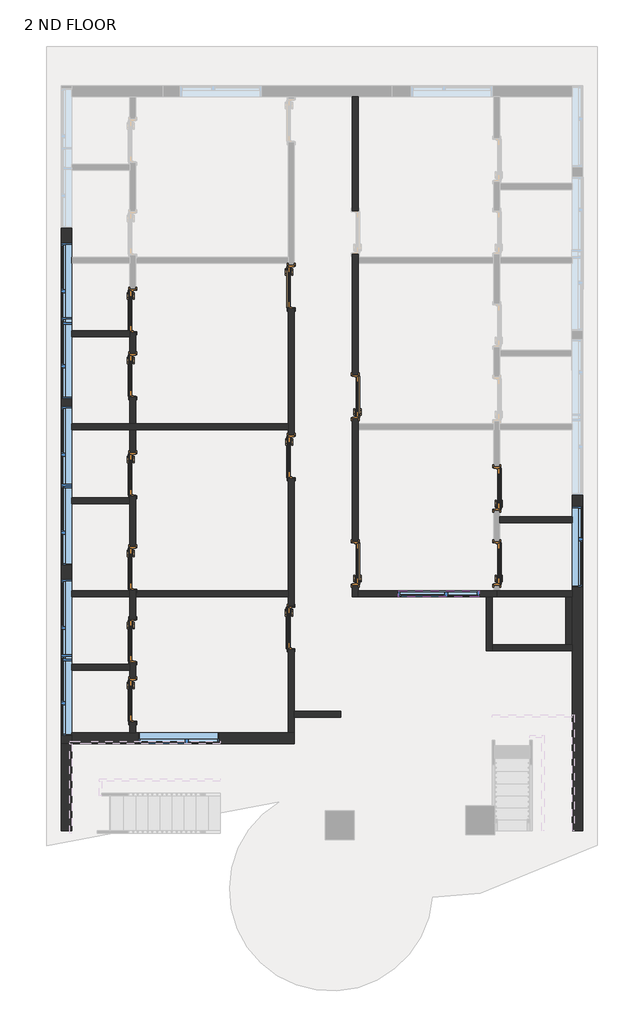
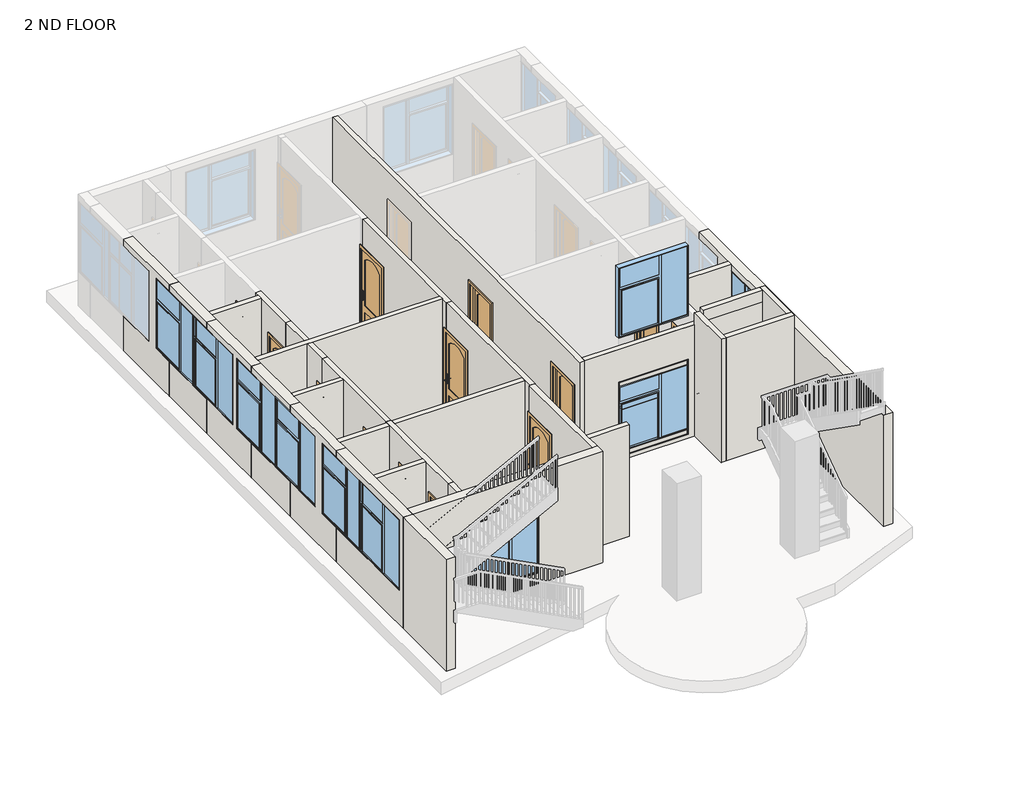
# One storey, part 1 of 4: 32 walls, 13 doors, 11 windows.
"""IFC4 building model written with IfcOpenShell, lengths in millimetres."""

from ifc_helpers import new_model, si_unit, frame, origin, place, context, project, spatial, polyline, outline, extrude, faceted_brep, transform, mapped, element, save
from components import door_346b4a94, m_window_casement_double_sidelight_1702_x_1829mm_c8b42c7f, m_window_casement_double_sidelight_1702_x_1829mm_92594323

model = new_model("IFC4")

# Units and contexts
model_context = context("Model", 3, world=origin())
ifc_project = project(units=[si_unit("LENGTHUNIT", "METRE", prefix="MILLI")], contexts=[model_context])

# Site, building, storey
site = spatial("IfcSite", under=ifc_project)
building = spatial("IfcBuilding", under=site)
storey = spatial("IfcBuildingStorey", under=building, Name="2 ND FLOOR", Elevation=6400.8)

# Doors
placement = place(None, origin())
door_shape = door_346b4a94(model_context)
element("IfcDoor", 1, ObjectType="2'10\"X7'", at=placement, inside=storey, context=model_context, shape_type="MappedRepresentation", body=[
    mapped(door_shape, transform((2698.7641134, -459.3600272, 6400.8), x_axis=(0.0, -1.0, 0.0), y_axis=(1.0, 0.0, 0.0), z_axis=(0.0, 0.0, 1.0))),
])
element("IfcDoor", 2, ObjectType="2'10\"X7'", at=placement, inside=storey, context=model_context, shape_type="MappedRepresentation", body=[
    mapped(door_shape, transform((2698.7641134, -2034.1600272, 6400.8), x_axis=(0.0, -1.0, 0.0), y_axis=(1.0, 0.0, 0.0), z_axis=(0.0, 0.0, 1.0))),
])
element("IfcDoor", 3, ObjectType="2'10\"X7'", at=placement, inside=storey, context=model_context, shape_type="MappedRepresentation", body=[
    mapped(door_shape, transform((-273.0358866, -2034.1600272, 6400.8), x_axis=(0.0, -1.0, 0.0), y_axis=(1.0, 0.0, 0.0), z_axis=(0.0, 0.0, 1.0))),
])
element("IfcDoor", 4, ObjectType="2'10\"X7'", at=placement, inside=storey, context=model_context, shape_type="MappedRepresentation", body=[
    mapped(door_shape, transform((-273.0358866, 1471.0399728, 6400.8), x_axis=(0.0, -1.0, 0.0), y_axis=(1.0, 0.0, 0.0), z_axis=(0.0, 0.0, 1.0))),
])
element("IfcDoor", 5, ObjectType="2'10\"X7'", at=placement, inside=storey, context=model_context, shape_type="MappedRepresentation", body=[
    mapped(door_shape, transform((-4952.9858866, -3659.7600272, 6400.8), x_axis=(0.0, 1.0, 0.0), y_axis=(-1.0, 0.0, 0.0), z_axis=(0.0, 0.0, 1.0))),
])
element("IfcDoor", 6, ObjectType="2'10\"X7'", at=placement, inside=storey, context=model_context, shape_type="MappedRepresentation", body=[
    mapped(door_shape, transform((-4952.9858866, -2142.5151651, 6400.8), x_axis=(0.0, 1.0, 0.0), y_axis=(-1.0, 0.0, 0.0), z_axis=(0.0, 0.0, 1.0))),
])
element("IfcDoor", 7, ObjectType="2'10\"X7'", at=placement, inside=storey, context=model_context, shape_type="MappedRepresentation", body=[
    mapped(door_shape, transform((-4952.9858866, -167.9704957, 6400.8), x_axis=(0.0, 1.0, 0.0), y_axis=(-1.0, 0.0, 0.0), z_axis=(0.0, 0.0, 1.0))),
])
element("IfcDoor", 8, ObjectType="2'10\"X7'", at=placement, inside=storey, context=model_context, shape_type="MappedRepresentation", body=[
    mapped(door_shape, transform((-4952.9858866, 3273.6174518, 6400.8), x_axis=(0.0, 1.0, 0.0), y_axis=(-1.0, 0.0, 0.0), z_axis=(0.0, 0.0, 1.0))),
])
element("IfcDoor", 9, ObjectType="2'10\"X7'", at=placement, inside=storey, context=model_context, shape_type="MappedRepresentation", body=[
    mapped(door_shape, transform((-1625.1621817, 3775.8008884, 6400.8), x_axis=(0.0, 1.0, 0.0), y_axis=(-1.0, 0.0, 0.0), z_axis=(0.0, 0.0, 1.0))),
])
element("IfcDoor", 10, ObjectType="2'10\"X7'", at=placement, inside=storey, context=model_context, shape_type="MappedRepresentation", body=[
    mapped(door_shape, transform((-1629.1419858, -3390.4626067, 6400.8), x_axis=(0.0, 1.0, 0.0), y_axis=(-1.0, 0.0, 0.0), z_axis=(0.0, 0.0, 1.0))),
])
element("IfcDoor", 11, ObjectType="2'10\"X7'", at=placement, inside=storey, context=model_context, shape_type="MappedRepresentation", body=[
    mapped(door_shape, transform((-1620.1577262, 202.9637706, 6400.8), x_axis=(0.0, 1.0, 0.0), y_axis=(-1.0, 0.0, 0.0), z_axis=(0.0, 0.0, 1.0))),
])
element("IfcDoor", 12, ObjectType="2'10\"X7'", at=placement, inside=storey, context=model_context, shape_type="MappedRepresentation", body=[
    mapped(door_shape, transform((-4952.9858866, -4917.0600272, 6400.8), x_axis=(0.0, 1.0, 0.0), y_axis=(-1.0, 0.0, 0.0), z_axis=(0.0, 0.0, 1.0))),
])
element("IfcDoor", 13, ObjectType="2'10\"X7'", at=placement, inside=storey, context=model_context, shape_type="MappedRepresentation", body=[
    mapped(door_shape, transform((-4952.9858866, 1913.3521609, 6400.8), x_axis=(0.0, 1.0, 0.0), y_axis=(-1.0, 0.0, 0.0), z_axis=(0.0, 0.0, 1.0))),
])

# Walls
element("IfcWall", 14, ObjectType="Generic - 4.5\"", at=placement, inside=storey, context=model_context, shape_type="Brep", body=[
    faceted_brep([(-6232.5508078, 2728.3399728, 6400.8), (-5013.3108866, 2728.3399728, 6400.8), (-5013.3108866, 2728.3399728, 9296.4), (-6232.5508078, 2728.3399728, 9296.4), (-6232.5508078, 2855.3399728, 6400.8), (-6232.5508078, 2855.3399728, 9296.4), (-5013.3108866, 2855.3399728, 9296.4), (-5013.3108866, 2855.3399728, 6400.8), (-5013.3108866, 2816.8174518, 6400.8)], [[[0, 1, 2, 3]], [[4, 5, 6, 7]], [[1, 0, 4, 7, 8]], [[0, 3, 5, 4]], [[2, 1, 8, 7, 6]], [[3, 2, 6, 5]]]),
])
element("IfcWall", 15, ObjectType="Generic - 4.5\"", at=placement, inside=storey, context=model_context, shape_type="Brep", body=[
    faceted_brep([(-5013.3108866, 2968.8174518, 9296.4), (-5013.3108866, 2968.8174518, 8559.4), (-5013.3108866, 2816.8174518, 8559.4), (-5013.3108866, 2816.8174518, 6400.8), (-5013.3108866, 2728.3399728, 6400.8), (-5013.3108866, 2370.1521609, 6400.8), (-5013.3108866, 2370.1521609, 8559.4), (-5013.3108866, 1684.7521609, 8559.4), (-5013.3108866, 1684.7521609, 9296.4), (-5013.3108866, 2728.3399728, 9296.4), (-5013.3108866, 2855.3399728, 9296.4), (-4886.3108866, 2968.8174518, 8559.4), (-4886.3108866, 2968.8174518, 9296.4), (-4886.3108866, 1684.7521609, 9296.4), (-4886.3108866, 1684.7521609, 8559.4), (-4886.3108866, 2370.1521609, 8559.4), (-4886.3108866, 2370.1521609, 6400.8), (-4886.3108866, 2816.8174518, 6400.8), (-4886.3108866, 2816.8174518, 8559.4)], [[[0, 1, 2, 3, 4, 5, 6, 7, 8, 9, 10]], [[11, 12, 13, 14, 15, 16, 17, 18]], [[3, 17, 16, 5, 4]], [[13, 8, 7, 14]], [[1, 0, 12, 11]], [[18, 2, 1, 11]], [[2, 18, 17, 3]], [[15, 6, 5, 16]], [[6, 15, 14, 7]], [[0, 10, 9, 8, 13, 12]]]),
])
element("IfcWall", 16, ObjectType="Generic - 4.5\"", at=placement, inside=storey, context=model_context, shape_type="Brep", body=[
    faceted_brep([(-6232.5508078, 772.5399728, 6400.8), (-5013.3108866, 772.5399728, 6400.8), (-4886.3108866, 772.5399728, 6400.8), (-1685.9108866, 772.5399728, 6400.8), (-1685.9108866, 772.5399728, 9296.4), (-4886.3108866, 772.5399728, 9296.4), (-5013.3108866, 772.5399728, 9296.4), (-6232.5508078, 772.5399728, 9296.4), (-6232.5508078, 899.5399728, 6400.8), (-6232.5508078, 899.5399728, 9296.4), (-5013.3108866, 899.5399728, 9296.4), (-4886.3108866, 899.5399728, 9296.4), (-1685.9108866, 899.5399728, 9296.4), (-1685.9108866, 899.5399728, 6400.8), (-4886.3108866, 899.5399728, 6400.8), (-5013.3108866, 899.5399728, 6400.8)], [[[0, 1, 2, 3, 4, 5, 6, 7]], [[8, 9, 10, 11, 12, 13, 14, 15]], [[3, 2, 1, 0, 8, 15, 14, 13]], [[4, 3, 13, 12]], [[0, 7, 9, 8]], [[7, 6, 5, 4, 12, 11, 10, 9]]]),
])
element("IfcWall", 17, ObjectType="Generic - 4.5\"", at=placement, inside=storey, context=model_context, shape_type="SweptSolid", body=[
    extrude(outline(polyline([(136.8295043, 8559.4), (136.8295043, 9296.4), (772.5399728, 9296.4), (772.5399728, 6400.8), (288.8295043, 6400.8), (288.8295043, 8559.4), (136.8295043, 8559.4)])), frame((-5013.3108866, 0.0, 0.0), z_axis=(1.0, 0.0, 0.0), x_axis=(0.0, 1.0, 0.0)), (0.0, 0.0, 1.0), 127.0),
    extrude(outline(polyline([(1684.7521609, 9296.4), (1684.7521609, 8559.4), (1456.5521609, 8559.4), (1456.5521609, 6400.8), (899.5399728, 6400.8), (899.5399728, 9296.4), (1684.7521609, 9296.4)])), frame((-5013.3108866, 0.0, 0.0), z_axis=(1.0, 0.0, 0.0), x_axis=(0.0, 1.0, 0.0)), (0.0, 0.0, 1.0), 127.0),
])
element("IfcWall", 18, ObjectType="Generic - 4.5\"", at=placement, inside=storey, context=model_context, shape_type="SweptSolid", body=[
    extrude(outline(polyline([(-5013.3108866, -776.8600272), (-6232.5508078, -776.8600272), (-6232.5508078, -649.8600272), (-5013.3108866, -649.8600272), (-5013.3108866, -776.8600272)])), frame((0.0, 0.0, 6400.8), z_axis=(0.0, 0.0, 1.0), x_axis=(1.0, 0.0, 0.0)), (0.0, 0.0, 1.0), 2895.6),
])
element("IfcWall", 19, ObjectType="Generic - 4.5\"", at=placement, inside=storey, context=model_context, shape_type="Brep", body=[
    faceted_brep([(-5013.3108866, -2574.3151651, 8559.4), (-5013.3108866, -2574.3151651, 9296.4), (-5013.3108866, -776.8600272, 9296.4), (-5013.3108866, -649.8600272, 9296.4), (-5013.3108866, 136.8295043, 9296.4), (-5013.3108866, 136.8295043, 8559.4), (-5013.3108866, -624.7704957, 8559.4), (-5013.3108866, -624.7704957, 6400.8), (-5013.3108866, -649.8600272, 6400.8), (-5013.3108866, -776.8600272, 6400.8), (-5013.3108866, -1685.7151651, 6400.8), (-5013.3108866, -1685.7151651, 8559.4), (-4886.3108866, -2574.3151651, 9296.4), (-4886.3108866, -2574.3151651, 8559.4), (-4886.3108866, -1685.7151651, 8559.4), (-4886.3108866, -1685.7151651, 6400.8), (-4886.3108866, -624.7704957, 6400.8), (-4886.3108866, -624.7704957, 8559.4), (-4886.3108866, 136.8295043, 8559.4), (-4886.3108866, 136.8295043, 9296.4)], [[[0, 1, 2, 3, 4, 5, 6, 7, 8, 9, 10, 11]], [[12, 13, 14, 15, 16, 17, 18, 19]], [[15, 10, 9, 8, 7, 16]], [[1, 0, 13, 12]], [[4, 19, 18, 5]], [[14, 11, 10, 15]], [[11, 14, 13, 0]], [[17, 6, 5, 18]], [[6, 17, 16, 7]], [[4, 3, 2, 1, 12, 19]]]),
])
element("IfcWall", 20, ObjectType="Generic - 4.5\"", at=placement, inside=storey, context=model_context, shape_type="SweptSolid", body=[
    extrude(outline(polyline([(-5013.3108866, -2732.6600272), (-6232.5508078, -2732.6600272), (-6232.5508078, -2605.6600272), (-5013.3108866, -2605.6600272), (-5013.3108866, -2732.6600272)])), frame((0.0, 0.0, 6400.8), z_axis=(0.0, 0.0, 1.0), x_axis=(1.0, 0.0, 0.0)), (0.0, 0.0, 1.0), 2895.6),
])
element("IfcWall", 21, ObjectType="Generic - 4.5\"", at=placement, inside=storey, context=model_context, shape_type="Brep", body=[
    faceted_brep([(-5013.3108866, -3202.9600272, 6400.8), (-5013.3108866, -3202.9600272, 8559.4), (-5013.3108866, -4116.5600272, 8559.4), (-5013.3108866, -4116.5600272, 6400.8), (-5013.3108866, -4155.0600272, 6400.8), (-5013.3108866, -4282.0600272, 6400.8), (-5013.3108866, -4460.2600272, 6400.8), (-5013.3108866, -4460.2600272, 8559.4), (-5013.3108866, -5221.8600272, 8559.4), (-5013.3108866, -5221.8600272, 9296.4), (-5013.3108866, -4282.0600272, 9296.4), (-5013.3108866, -4155.0600272, 9296.4), (-5013.3108866, -2732.6600272, 9296.4), (-5013.3108866, -2605.6600272, 9296.4), (-5013.3108866, -2574.3151651, 9296.4), (-5013.3108866, -2574.3151651, 8559.4), (-5013.3108866, -2599.3151651, 8559.4), (-5013.3108866, -2599.3151651, 6400.8), (-5013.3108866, -2605.6600272, 6400.8), (-5013.3108866, -2732.6600272, 6400.8), (-4886.3108866, -3202.9600272, 8559.4), (-4886.3108866, -3202.9600272, 6400.8), (-4886.3108866, -2732.6600272, 6400.8), (-4886.3108866, -2605.6600272, 6400.8), (-4886.3108866, -2599.3151651, 6400.8), (-4886.3108866, -2599.3151651, 8559.4), (-4886.3108866, -2574.3151651, 8559.4), (-4886.3108866, -2574.3151651, 9296.4), (-4886.3108866, -2605.6600272, 9296.4), (-4886.3108866, -2732.6600272, 9296.4), (-4886.3108866, -5221.8600272, 9296.4), (-4886.3108866, -5221.8600272, 8559.4), (-4886.3108866, -4460.2600272, 8559.4), (-4886.3108866, -4460.2600272, 6400.8), (-4886.3108866, -4116.5600272, 6400.8), (-4886.3108866, -4116.5600272, 8559.4)], [[[0, 1, 2, 3, 4, 5, 6, 7, 8, 9, 10, 11, 12, 13, 14, 15, 16, 17, 18, 19]], [[20, 21, 22, 23, 24, 25, 26, 27, 28, 29, 30, 31, 32, 33, 34, 35]], [[21, 0, 19, 18, 17, 24, 23, 22]], [[3, 34, 33, 6, 5, 4]], [[30, 9, 8, 31]], [[15, 14, 27, 26]], [[20, 1, 0, 21]], [[1, 20, 35, 2]], [[2, 35, 34, 3]], [[25, 16, 15, 26]], [[16, 25, 24, 17]], [[32, 7, 6, 33]], [[7, 32, 31, 8]], [[14, 13, 12, 11, 10, 9, 30, 29, 28, 27]]]),
])
element("IfcWall", 22, ObjectType="Generic - 4.5\"", at=placement, inside=storey, context=model_context, shape_type="SweptSolid", body=[
    extrude(outline(polyline([(-5013.3108866, -4282.0600272), (-6232.5324766, -4282.0600272), (-6232.5342541, -4155.0600272), (-5013.3108866, -4155.0600272), (-5013.3108866, -4282.0600272)])), frame((0.0, 0.0, 6400.8), z_axis=(0.0, 0.0, 1.0), x_axis=(1.0, 0.0, 0.0)), (0.0, 0.0, 1.0), 2895.6),
])
element("IfcWall", 23, ObjectType="Generic - 4.5\"", at=placement, inside=storey, context=model_context, shape_type="SweptSolid", body=[
    extrude(outline(polyline([(-1685.9108866, -2732.6600272), (-4886.3108866, -2732.6600272), (-4886.3108866, -2605.6600272), (-1685.9108866, -2605.6600272), (-1685.9108866, -2732.6600272)])), frame((0.0, 0.0, 6400.8), z_axis=(0.0, 0.0, 1.0), x_axis=(1.0, 0.0, 0.0)), (0.0, 0.0, 1.0), 2895.6),
])
element("IfcWall", 24, ObjectType="Generic - 4.5\"", at=placement, inside=storey, context=model_context, shape_type="Brep", body=[
    faceted_brep([(-1685.4871817, 4182.2008884, 9296.4), (-1685.4871817, 4182.2008884, 8559.4), (-1685.4871817, 3319.0008884, 8559.4), (-1685.4871817, 3319.0008884, 6400.8), (-1685.4871817, 659.7637706, 6400.8), (-1685.4871817, 659.7637706, 8559.4), (-1685.4871817, 609.3637706, 8559.4), (-1685.4871817, 609.3637706, 9296.4), (-1558.4871817, 4182.2008884, 8559.4), (-1558.4871817, 4182.2008884, 9296.4), (-1558.4871817, 609.3637706, 9296.4), (-1558.4871817, 609.3637706, 8559.4), (-1558.4871817, 659.7637706, 8559.4), (-1558.4871817, 659.7637706, 6400.8), (-1558.4871817, 3319.0008884, 6400.8), (-1558.4871817, 3319.0008884, 8559.4), (-1680.4827262, 609.3637706, 9296.4), (-1680.4827262, 609.3637706, 8559.4), (-1558.9108866, 4182.2008884, 9296.4), (-1558.9108866, 4182.2008884, 8559.4)], [[[0, 1, 2, 3, 4, 5, 6, 7]], [[8, 9, 10, 11, 12, 13, 14, 15]], [[3, 14, 13, 4]], [[10, 16, 7, 6, 17, 11]], [[1, 0, 18, 9, 8, 19]], [[15, 2, 1, 19, 8]], [[2, 15, 14, 3]], [[12, 5, 4, 13]], [[5, 12, 11, 17, 6]], [[0, 7, 16, 10, 9, 18]]]),
])
element("IfcWall", 25, ObjectType="Generic - 4.5\"", at=placement, inside=storey, context=model_context, shape_type="Brep", body=[
    faceted_brep([(-1680.4827262, -2933.2626067, 6400.8), (-1680.4827262, -2933.2626067, 9296.4), (-1680.4827262, 609.3637706, 9296.4), (-1680.4827262, 609.3637706, 8559.4), (-1680.4827262, -253.8362294, 8559.4), (-1680.4827262, -253.8362294, 6400.8), (-1553.4827262, -2933.2626067, 9296.4), (-1553.4827262, -2933.2626067, 6400.8), (-1553.4827262, -253.8362294, 6400.8), (-1553.4827262, -253.8362294, 8559.4), (-1553.4827262, 609.3637706, 8559.4), (-1553.4827262, 609.3637706, 9296.4), (-1562.4669858, -2933.2626067, 6400.8), (-1562.4669858, -2933.2626067, 9296.4), (-1558.4871817, 609.3637706, 9296.4), (-1558.4871817, 609.3637706, 8559.4)], [[[0, 1, 2, 3, 4, 5]], [[6, 7, 8, 9, 10, 11]], [[7, 12, 0, 5, 8]], [[1, 0, 12, 7, 6, 13]], [[2, 14, 11, 10, 15, 3]], [[9, 4, 3, 15, 10]], [[4, 9, 8, 5]], [[2, 1, 13, 6, 11, 14]]]),
])
element("IfcWall", 26, ObjectType="Generic - 4.5\"", at=placement, inside=storey, context=model_context, shape_type="Brep", body=[
    faceted_brep([(-1689.4669858, -2933.2626067, 9296.4), (-1689.4669858, -2933.2626067, 6400.8), (-1689.4669858, -2933.6626067, 6400.8), (-1689.4669858, -2933.6626067, 8559.4), (-1689.4669858, -3847.2626067, 8559.4), (-1689.4669858, -3847.2626067, 6400.8), (-1689.4669858, -5596.1082131, 6400.8), (-1689.4669858, -5596.1082131, 9296.4), (-1562.4669858, -2933.2626067, 6400.8), (-1562.4669858, -2933.2626067, 9296.4), (-1562.4669858, -5136.3822004, 9296.4), (-1562.4669858, -5263.3822004, 9296.4), (-1562.4669858, -5596.1082131, 9296.4), (-1562.4669858, -5596.1082131, 6400.8), (-1562.4669858, -5263.3822004, 6400.8), (-1562.4669858, -5136.3822004, 6400.8), (-1562.4669858, -3847.2626067, 6400.8), (-1562.4669858, -3847.2626067, 8559.4), (-1562.4669858, -2933.6626067, 8559.4), (-1562.4669858, -2933.6626067, 6400.8), (-1680.4827262, -2933.2626067, 6400.8), (-1680.4827262, -2933.2626067, 9296.4)], [[[0, 1, 2, 3, 4, 5, 6, 7]], [[8, 9, 10, 11, 12, 13, 14, 15, 16, 17, 18, 19]], [[1, 20, 8, 19, 2]], [[13, 6, 5, 16, 15, 14]], [[1, 0, 21, 9, 8, 20]], [[18, 3, 2, 19]], [[3, 18, 17, 4]], [[4, 17, 16, 5]], [[7, 6, 13, 12]], [[0, 7, 12, 11, 10, 9, 21]]]),
])
element("IfcWall", 27, ObjectType="Generic - 4.5\"", at=placement, inside=storey, context=model_context, shape_type="Brep", body=[
    faceted_brep([(-339.7108866, 7782.9399728, 9296.4), (-339.7108866, 7782.9399728, 6400.8), (-339.7108866, 5382.2399728, 6400.8), (-339.7108866, 5382.2399728, 8559.4), (-339.7108866, 4468.6399728, 8559.4), (-339.7108866, 4468.6399728, 6400.8), (-339.7108866, 1927.8399728, 6400.8), (-339.7108866, 1927.8399728, 8559.4), (-339.7108866, 1014.2399728, 8559.4), (-339.7108866, 1014.2399728, 6400.8), (-339.7108866, -1577.3600272, 6400.8), (-339.7108866, -1577.3600272, 8559.4), (-339.7108866, -2490.9600272, 8559.4), (-339.7108866, -2490.9600272, 6400.8), (-339.7108866, -2732.6600272, 6400.8), (-339.7108866, -2732.6600272, 9296.4), (-212.7108866, 7782.9399728, 6400.8), (-212.7108866, 7782.9399728, 9296.4), (-212.7108866, 4404.7399728, 9296.4), (-212.7108866, 4277.7399728, 9296.4), (-212.7108866, 899.5399728, 9296.4), (-212.7108866, 772.5399728, 9296.4), (-212.7108866, -2605.6600272, 9296.4), (-212.7108866, -2732.6600272, 9296.4), (-212.7108866, -2732.6600272, 6400.8), (-212.7108866, -2605.6600272, 6400.8), (-212.7108866, -2490.9600272, 6400.8), (-212.7108866, -2490.9600272, 8559.4), (-212.7108866, -1577.3600272, 8559.4), (-212.7108866, -1577.3600272, 6400.8), (-212.7108866, 772.5399728, 6400.8), (-212.7108866, 899.5399728, 6400.8), (-212.7108866, 1014.2399728, 6400.8), (-212.7108866, 1014.2399728, 8559.4), (-212.7108866, 1927.8399728, 8559.4), (-212.7108866, 1927.8399728, 6400.8), (-212.7108866, 4277.7399728, 6400.8), (-212.7108866, 4404.7399728, 6400.8), (-212.7108866, 4468.6399728, 6400.8), (-212.7108866, 4468.6399728, 8559.4), (-212.7108866, 5382.2399728, 8559.4), (-212.7108866, 5382.2399728, 6400.8)], [[[0, 1, 2, 3, 4, 5, 6, 7, 8, 9, 10, 11, 12, 13, 14, 15]], [[16, 17, 18, 19, 20, 21, 22, 23, 24, 25, 26, 27, 28, 29, 30, 31, 32, 33, 34, 35, 36, 37, 38, 39, 40, 41]], [[1, 16, 41, 2]], [[24, 14, 13, 26, 25]], [[29, 10, 9, 32, 31, 30]], [[35, 6, 5, 38, 37, 36]], [[1, 0, 17, 16]], [[15, 14, 24, 23]], [[12, 27, 26, 13]], [[27, 12, 11, 28]], [[28, 11, 10, 29]], [[8, 33, 32, 9]], [[33, 8, 7, 34]], [[34, 7, 6, 35]], [[4, 39, 38, 5]], [[39, 4, 3, 40]], [[40, 3, 2, 41]], [[0, 15, 23, 22, 21, 20, 19, 18, 17]]]),
])
element("IfcWall", 28, ObjectType="Generic - 4.5\"", at=placement, inside=storey, context=model_context, shape_type="Brep", body=[
    faceted_brep([(-212.7108866, -2732.6600272, 6400.8), (2479.6891134, -2732.6600272, 6400.8), (2606.6891134, -2732.6600272, 6400.8), (4281.7311655, -2732.6600272, 6400.8), (4281.7311655, -2732.6600272, 9296.4), (-212.7108866, -2732.6600272, 9296.4), (625.4891134, -2732.6600272, 8454.7930467), (2327.2891134, -2732.6600272, 8454.7930467), (2327.2891134, -2732.6600272, 6625.9930467), (625.4891134, -2732.6600272, 6625.9930467), (-212.7108866, -2605.6600272, 6400.8), (-212.7108866, -2605.6600272, 9296.4), (2632.0891134, -2605.6600272, 9296.4), (2759.0891134, -2605.6600272, 9296.4), (4281.7311655, -2605.6600272, 9296.4), (4281.7311655, -2605.6600272, 6400.8), (2759.0891134, -2605.6600272, 6400.8), (2632.0891134, -2605.6600272, 6400.8), (625.4891134, -2605.6600272, 8454.7930467), (625.4891134, -2605.6600272, 6625.9930467), (2327.2891134, -2605.6600272, 6625.9930467), (2327.2891134, -2605.6600272, 8454.7930467)], [[[0, 1, 2, 3, 4, 5], [6, 7, 8, 9]], [[10, 11, 12, 13, 14, 15, 16, 17], [18, 19, 20, 21]], [[3, 2, 1, 0, 10, 17, 16, 15]], [[0, 5, 11, 10]], [[4, 3, 15, 14]], [[5, 4, 14, 13, 12, 11]], [[19, 18, 6, 9]], [[20, 19, 9, 8]], [[21, 20, 8, 7]], [[18, 21, 7, 6]]]),
])
element("IfcWall", 29, ObjectType="Generic - 4.5\"", at=placement, inside=storey, context=model_context, shape_type="SweptSolid", body=[
    extrude(outline(polyline([(4281.7311655, -1183.2600272), (2759.0891134, -1183.2600272), (2759.0891134, -1056.2600272), (4281.7311655, -1056.2600272), (4281.7311655, -1183.2600272)])), frame((0.0, 0.0, 6400.8), z_axis=(0.0, 0.0, 1.0), x_axis=(1.0, 0.0, 0.0)), (0.0, 0.0, 1.0), 2895.6),
])
element("IfcWall", 30, ObjectType="Generic - 4.5\"", at=placement, inside=storey, context=model_context, shape_type="Brep", body=[
    faceted_brep([(-212.7108866, -2732.6600272, 6400.8), (2479.6891134, -2732.6600272, 6400.8), (2606.6891134, -2732.6600272, 6400.8), (2695.5891134, -2732.6600272, 6400.8), (2695.5891134, -2732.6600272, 9296.4), (-212.7108866, -2732.6600272, 9296.4), (625.4891134, -2732.6600272, 8326.7883506), (2327.2891134, -2732.6600272, 8326.7883506), (2327.2891134, -2732.6600272, 6497.9883506), (625.4891134, -2732.6600272, 6497.9883506), (-212.7108866, -2605.6600272, 6400.8), (-212.7108866, -2605.6600272, 9296.4), (2632.0891134, -2605.6600272, 9296.4), (2695.5891134, -2605.6600272, 9296.4), (2695.5891134, -2605.6600272, 6400.8), (2632.0891134, -2605.6600272, 6400.8), (625.4891134, -2605.6600272, 8326.7883506), (625.4891134, -2605.6600272, 6497.9883506), (2327.2891134, -2605.6600272, 6497.9883506), (2327.2891134, -2605.6600272, 8326.7883506)], [[[0, 1, 2, 3, 4, 5], [6, 7, 8, 9]], [[10, 11, 12, 13, 14, 15], [16, 17, 18, 19]], [[3, 2, 1, 0, 10, 15, 14]], [[4, 3, 14, 13]], [[5, 4, 13, 12, 11]], [[17, 16, 6, 9]], [[18, 17, 9, 8]], [[19, 18, 8, 7]], [[16, 19, 7, 6]], [[0, 5, 11, 10]]]),
])
element("IfcWall", 31, ObjectType="Generic - 5\"", at=placement, inside=storey, context=model_context, shape_type="SweptSolid", body=[
    extrude(outline(polyline([(-5593.5822004, 6400.8), (-5593.5822004, 9296.4), (-5221.8600272, 9296.4), (-5221.8600272, 8559.4), (-5373.8600272, 8559.4), (-5373.8600272, 6400.8), (-5593.5822004, 6400.8)])), frame((-5013.3108866, 0.0, 0.0), z_axis=(1.0, 0.0, 0.0), x_axis=(0.0, 1.0, 0.0)), (0.0, 0.0, 1.0), 127.0),
])
element("IfcWall", 32, ObjectType="Generic - 5\"", at=placement, inside=storey, context=model_context, shape_type="SweptSolid", body=[
    extrude(outline(polyline([(-1562.4669858, -5136.3822004), (-581.0108866, -5136.3822004), (-581.0108866, -5263.3822004), (-1562.4669858, -5263.3822004), (-1562.4669858, -5136.3822004)])), frame((0.0, 0.0, 6400.8), z_axis=(0.0, 0.0, 1.0), x_axis=(1.0, 0.0, 0.0)), (0.0, 0.0, 1.0), 2895.6),
])
element("IfcWall", 33, ObjectType="Generic - 5\"", at=placement, inside=storey, context=model_context, shape_type="Brep", body=[
    faceted_brep([(2479.6891134, -2732.6600272, 6400.8), (2479.6891134, -3866.3822004, 6400.8), (2479.6891134, -3866.3822004, 9601.2), (2479.6891134, -2732.6600272, 9601.2), (2606.6891134, -2732.6600272, 6400.8), (2606.6891134, -2732.6600272, 9601.2), (2606.6891134, -3739.3822004, 9601.2), (2606.6891134, -3866.3822004, 9601.2), (2606.6891134, -3866.3822004, 6400.8), (2606.6891134, -3739.3822004, 6400.8)], [[[0, 1, 2, 3]], [[4, 5, 6, 7, 8, 9]], [[1, 0, 4, 9, 8]], [[3, 2, 7, 6, 5]], [[0, 3, 5, 4]], [[2, 1, 8, 7]]]),
])
element("IfcWall", 34, ObjectType="Generic - 5\"", at=placement, inside=storey, context=model_context, shape_type="Brep", body=[
    faceted_brep([(2606.6891134, -3866.3822004, 6400.8), (4281.7311655, -3866.3822004, 6400.8), (4281.7311655, -3866.3822004, 9601.2), (2606.6891134, -3866.3822004, 9601.2), (2606.6891134, -3739.3822004, 6400.8), (2606.6891134, -3739.3822004, 9601.2), (4154.7311655, -3739.3822004, 9601.2), (4281.7311655, -3739.3822004, 9601.2), (4281.7311655, -3739.3822004, 6400.8), (4154.7311655, -3739.3822004, 6400.8)], [[[0, 1, 2, 3]], [[4, 5, 6, 7, 8, 9]], [[1, 0, 4, 9, 8]], [[3, 2, 7, 6, 5]], [[0, 3, 5, 4]], [[2, 1, 8, 7]]]),
])
element("IfcWall", 35, ObjectType="Generic - 5\"", at=placement, inside=storey, context=model_context, shape_type="Brep", body=[
    faceted_brep([(4281.7311655, -3739.3822004, 6400.8), (4281.7311655, -2605.6600272, 6400.8), (4281.7311655, -2605.6600272, 9601.2), (4281.7311655, -3739.3822004, 9601.2), (4154.7311655, -3739.3822004, 6400.8), (4154.7311655, -3739.3822004, 9601.2), (4154.7311655, -2732.6600272, 9601.2), (4154.7311655, -2605.6600272, 9601.2), (4154.7311655, -2605.6600272, 6400.8), (4154.7311655, -2732.6600272, 6400.8)], [[[0, 1, 2, 3]], [[4, 5, 6, 7, 8, 9]], [[1, 0, 4, 9, 8]], [[3, 2, 7, 6, 5]], [[0, 3, 5, 4]], [[1, 8, 7, 2]]]),
])
element("IfcWall", 36, ObjectType="Generic - 5\"", at=placement, inside=storey, context=model_context, shape_type="Brep", body=[
    faceted_brep([(2695.5891134, -2732.6600272, 6400.8), (4154.7311655, -2732.6600272, 6400.8), (4154.7311655, -2732.6600272, 9601.2), (2695.5891134, -2732.6600272, 9601.2), (2695.5891134, -2732.6600272, 9296.4), (2695.5891134, -2605.6600272, 6400.8), (2695.5891134, -2605.6600272, 9296.4), (2695.5891134, -2605.6600272, 9601.2), (4154.7311655, -2605.6600272, 9601.2), (4154.7311655, -2605.6600272, 6400.8), (2759.0891134, -2605.6600272, 6400.8)], [[[0, 1, 2, 3, 4]], [[5, 6, 7, 8, 9, 10]], [[1, 0, 5, 10, 9]], [[3, 2, 8, 7]], [[0, 4, 3, 7, 6, 5]], [[2, 1, 9, 8]]]),
])
element("IfcWall", 37, ObjectType="Generic - 9\"", at=placement, inside=storey, context=model_context, shape_type="Brep", body=[
    faceted_brep([(4281.7311655, 200.5184135, 6400.8), (4281.7311655, -1056.2600272, 6400.8), (4281.7311655, -1183.2600272, 6400.8), (4281.7311655, -2605.6600272, 6400.8), (4281.7311655, -2732.6600272, 6400.8), (4281.7311655, -7650.9822004, 6400.8), (4281.7311655, -7650.9822004, 9296.4), (4281.7311655, -2732.6600272, 9296.4), (4281.7311655, -2605.6600272, 9296.4), (4281.7311655, -1183.2600272, 9296.4), (4281.7311655, -1056.2600272, 9296.4), (4281.7311655, 200.5184135, 9296.4), (4281.7311655, 200.5184135, 9129.6), (4281.7311655, -599.0600272, 9129.6), (4281.7311655, -599.0600272, 7300.8), (4281.7311655, 200.5184135, 7300.8), (4281.7311655, -2537.537179, 7300.8), (4281.7311655, -835.737179, 7300.8), (4281.7311655, -835.737179, 9129.6), (4281.7311655, -2537.537179, 9129.6), (4510.3311655, -7650.9822004, 6400.8), (4510.3311655, 200.5184135, 6400.8), (4510.3311655, 200.5184135, 7300.8), (4510.3311655, -599.0600272, 7300.8), (4510.3311655, -599.0600272, 9129.6), (4510.3311655, 200.5184135, 9129.6), (4510.3311655, 200.5184135, 9296.4), (4510.3311655, -7650.9822004, 9296.4), (4510.3311655, -835.737179, 7300.8), (4510.3311655, -2537.537179, 7300.8), (4510.3311655, -2537.537179, 9129.6), (4510.3311655, -835.737179, 9129.6), (4283.0918814, 200.5184135, 6400.8), (4283.0918814, 200.5184135, 7300.8), (4283.0918814, 200.5184135, 9296.4), (4283.0918814, 200.5184135, 9129.6)], [[[0, 1, 2, 3, 4, 5, 6, 7, 8, 9, 10, 11, 12, 13, 14, 15], [16, 17, 18, 19]], [[20, 21, 22, 23, 24, 25, 26, 27], [28, 29, 30, 31]], [[5, 4, 3, 2, 1, 0, 32, 21, 20]], [[6, 5, 20, 27]], [[21, 32, 0, 15, 33, 22]], [[12, 11, 34, 26, 25, 35]], [[13, 24, 23, 14]], [[14, 23, 22, 33, 15]], [[24, 13, 12, 35, 25]], [[28, 17, 16, 29]], [[17, 28, 31, 18]], [[18, 31, 30, 19]], [[29, 16, 19, 30]], [[11, 10, 9, 8, 7, 6, 27, 26, 34]]]),
])
element("IfcWall", 38, ObjectType="Generic - 9\"", at=placement, inside=storey, context=model_context, shape_type="Brep", body=[
    faceted_brep([(-6232.5108866, -5824.7082131, 6400.8), (-6232.5140859, -5596.1082131, 6400.8), (-6232.5324766, -4282.0600272, 6400.8), (-6232.5342541, -4155.0600272, 6400.8), (-6232.5508078, -2972.263382, 6400.8), (-6232.5508078, -2972.263382, 7300.8), (-6232.5131972, -5659.6082132, 7300.8), (-6232.5131972, -5659.6082132, 9129.6), (-6232.5508078, -2972.263382, 9129.6), (-6232.5508078, -2972.263382, 9296.4), (-6232.5342541, -4155.0600272, 9296.4), (-6232.5324766, -4282.0600272, 9296.4), (-6232.5140859, -5596.1082131, 9296.4), (-6232.5108866, -5824.7082131, 9296.4), (-6461.1508078, -2972.2665814, 6400.8), (-6461.1108866, -5824.7082131, 6400.8), (-6461.1108866, -5824.7082131, 9296.4), (-6461.1508078, -2972.2665814, 9296.4), (-6461.1508078, -2972.2665814, 9129.6), (-6461.1131972, -5659.6114126, 9129.6), (-6461.1131972, -5659.6114126, 7300.8), (-6461.1508078, -2972.2665814, 7300.8)], [[[0, 1, 2, 3, 4, 5, 6, 7, 8, 9, 10, 11, 12, 13]], [[14, 15, 16, 17, 18, 19, 20, 21]], [[4, 3, 2, 1, 0, 15, 14]], [[4, 14, 21, 5]], [[9, 8, 18, 17]], [[5, 21, 20, 6]], [[18, 8, 7, 19]], [[19, 7, 6, 20]], [[0, 13, 16, 15]], [[13, 12, 11, 10, 9, 17, 16]]]),
])
element("IfcWall", 39, ObjectType="Generic - 9\"", at=placement, inside=storey, context=model_context, shape_type="Brep", body=[
    faceted_brep([(-6232.5508078, -2972.2649817, 6400.8), (-6232.5508078, -2732.6600272, 6400.8), (-6232.5508078, -2605.6600272, 6400.8), (-6232.5508078, -1019.7048138, 6400.8), (-6232.5508078, -1019.7048138, 7300.8), (-6232.5508078, -2073.8048138, 7300.8), (-6232.5508078, -2073.8048138, 9129.6), (-6232.5508078, -1019.7048138, 9129.6), (-6232.5508078, -1019.7048138, 9296.4), (-6232.5508078, -2605.6600272, 9296.4), (-6232.5508078, -2732.6600272, 9296.4), (-6232.5508078, -2972.2649817, 9296.4), (-6232.5508078, -2972.2649817, 9129.6), (-6232.5508078, -2375.3633819, 9129.6), (-6232.5508078, -2375.3633819, 7300.8), (-6232.5508078, -2972.2649817, 7300.8), (-6461.1508078, -1019.7048138, 6400.8), (-6461.1508078, -2972.2649817, 6400.8), (-6461.1508078, -2972.2649817, 7300.8), (-6461.1508078, -2375.3665813, 7300.8), (-6461.1508078, -2375.3665813, 9129.6), (-6461.1508078, -2972.2649817, 9129.6), (-6461.1508078, -2972.2649817, 9296.4), (-6461.1508078, -1019.7048138, 9296.4), (-6461.1508078, -1019.7048138, 9129.6), (-6461.1508078, -2073.8048138, 9129.6), (-6461.1508078, -2073.8048138, 7300.8), (-6461.1508078, -1019.7048138, 7300.8)], [[[0, 1, 2, 3, 4, 5, 6, 7, 8, 9, 10, 11, 12, 13, 14, 15]], [[16, 17, 18, 19, 20, 21, 22, 23, 24, 25, 26, 27]], [[3, 2, 1, 0, 17, 16]], [[3, 16, 27, 4]], [[8, 7, 24, 23]], [[17, 0, 15, 18]], [[11, 22, 21, 12]], [[26, 5, 4, 27]], [[5, 26, 25, 6]], [[6, 25, 24, 7]], [[13, 20, 19, 14]], [[14, 19, 18, 15]], [[20, 13, 12, 21]], [[11, 10, 9, 8, 23, 22]]]),
])
element("IfcWall", 40, ObjectType="Generic - 9\"", at=placement, inside=storey, context=model_context, shape_type="Brep", body=[
    faceted_brep([(-6232.5508078, -1019.7048138, 6400.8), (-6232.5508078, -776.8600272, 6400.8), (-6232.5508078, -649.8600272, 6400.8), (-6232.5508078, 642.0011338, 6400.8), (-6232.5508078, 642.0011338, 7300.8), (-6232.5508078, -1019.7048138, 7300.8), (-6461.1508078, 642.0011338, 6400.8), (-6461.1508078, -1019.7048138, 6400.8), (-6461.1508078, -1019.7048138, 7300.8), (-6461.1508078, 642.0011338, 7300.8)], [[[0, 1, 2, 3, 4, 5]], [[6, 7, 8, 9]], [[3, 2, 1, 0, 7, 6]], [[3, 6, 9, 4]], [[7, 0, 5, 8]], [[4, 9, 8, 5]]]),
    faceted_brep([(-6232.5508078, -1019.7048138, 9129.6), (-6232.5508078, 642.0011338, 9129.6), (-6232.5508078, 642.0011338, 9296.4), (-6232.5508078, -649.8600272, 9296.4), (-6232.5508078, -776.8600272, 9296.4), (-6232.5508078, -1019.7048138, 9296.4), (-6461.1508078, 642.0011338, 9296.4), (-6461.1508078, 642.0011338, 9129.6), (-6461.1508078, -1019.7048138, 9129.6), (-6461.1508078, -1019.7048138, 9296.4)], [[[0, 1, 2, 3, 4, 5]], [[6, 7, 8, 9]], [[2, 1, 7, 6]], [[5, 9, 8, 0]], [[7, 1, 0, 8]], [[5, 4, 3, 2, 6, 9]]]),
])
element("IfcWall", 41, ObjectType="Generic - 9\"", at=placement, inside=storey, context=model_context, shape_type="Brep", body=[
    faceted_brep([(-6232.5508078, 642.0011338, 6400.8), (-6232.5508078, 772.5399728, 6400.8), (-6232.5508078, 899.5399728, 6400.8), (-6232.5508078, 2534.5107865, 6400.8), (-6232.5508078, 2534.5107865, 7300.8), (-6232.5508078, 1429.6107865, 7300.8), (-6232.5508078, 1429.6107865, 9129.6), (-6232.5508078, 2534.5107865, 9129.6), (-6232.5508078, 2534.5107865, 9296.4), (-6232.5508078, 899.5399728, 9296.4), (-6232.5508078, 772.5399728, 9296.4), (-6232.5508078, 642.0011338, 9296.4), (-6232.5508078, 642.0011338, 9129.6), (-6232.5508078, 1264.3011338, 9129.6), (-6232.5508078, 1264.3011338, 7300.8), (-6232.5508078, 642.0011338, 7300.8), (-6461.1508078, 2534.5107865, 6400.8), (-6461.1508078, 642.0011338, 6400.8), (-6461.1508078, 642.0011338, 7300.8), (-6461.1508078, 1264.3011338, 7300.8), (-6461.1508078, 1264.3011338, 9129.6), (-6461.1508078, 642.0011338, 9129.6), (-6461.1508078, 642.0011338, 9296.4), (-6461.1508078, 2534.5107865, 9296.4), (-6461.1508078, 2534.5107865, 9129.6), (-6461.1508078, 1429.6107865, 9129.6), (-6461.1508078, 1429.6107865, 7300.8), (-6461.1508078, 2534.5107865, 7300.8)], [[[0, 1, 2, 3, 4, 5, 6, 7, 8, 9, 10, 11, 12, 13, 14, 15]], [[16, 17, 18, 19, 20, 21, 22, 23, 24, 25, 26, 27]], [[3, 2, 1, 0, 17, 16]], [[3, 16, 27, 4]], [[8, 7, 24, 23]], [[17, 0, 15, 18]], [[11, 22, 21, 12]], [[26, 5, 4, 27]], [[5, 26, 25, 6]], [[6, 25, 24, 7]], [[13, 20, 19, 14]], [[14, 19, 18, 15]], [[20, 13, 12, 21]], [[11, 10, 9, 8, 23, 22]]]),
])
element("IfcWall", 42, ObjectType="Generic - 9\"", at=placement, inside=storey, context=model_context, shape_type="Brep", body=[
    faceted_brep([(-6232.5508078, 2534.5107865, 6400.8), (-6232.5508078, 2728.3399728, 6400.8), (-6232.5508078, 2855.3399728, 6400.8), (-6232.5508078, 4130.2388609, 6400.8), (-6232.5508078, 4130.2388609, 7300.8), (-6232.5508078, 2534.5107865, 7300.8), (-6461.1508078, 4130.2388609, 6400.8), (-6461.1508078, 2534.5107865, 6400.8), (-6461.1508078, 2534.5107865, 7300.8), (-6461.1508078, 4130.2388609, 7300.8)], [[[0, 1, 2, 3, 4, 5]], [[6, 7, 8, 9]], [[3, 2, 1, 0, 7, 6]], [[3, 6, 9, 4]], [[7, 0, 5, 8]], [[4, 9, 8, 5]]]),
    faceted_brep([(-6232.5508078, 2534.5107865, 9129.6), (-6232.5508078, 4130.2388609, 9129.6), (-6232.5508078, 4130.2388609, 9296.4), (-6232.5508078, 2855.3399728, 9296.4), (-6232.5508078, 2728.3399728, 9296.4), (-6232.5508078, 2534.5107865, 9296.4), (-6461.1508078, 4130.2388609, 9296.4), (-6461.1508078, 4130.2388609, 9129.6), (-6461.1508078, 2534.5107865, 9129.6), (-6461.1508078, 2534.5107865, 9296.4)], [[[0, 1, 2, 3, 4, 5]], [[6, 7, 8, 9]], [[2, 1, 7, 6]], [[5, 9, 8, 0]], [[7, 1, 0, 8]], [[5, 4, 3, 2, 6, 9]]]),
])
element("IfcWall", 43, ObjectType="Generic - 9\"", at=placement, inside=storey, context=model_context, shape_type="Brep", body=[
    faceted_brep([(-6232.5508078, 4130.2388609, 6400.8), (-6232.5508078, 4277.7399728, 6400.8), (-6232.5508078, 4404.7399728, 6400.8), (-6232.5508078, 6088.0863192, 6400.8), (-6232.5508078, 6088.0863192, 7300.8), (-6232.5508078, 5008.5863192, 7300.8), (-6232.5508078, 5008.5863192, 9129.6), (-6232.5508078, 6088.0863192, 9129.6), (-6232.5508078, 6088.0863192, 9296.4), (-6232.5508078, 4404.7399728, 9296.4), (-6232.5508078, 4277.7399728, 9296.4), (-6232.5508078, 4130.2388609, 9296.4), (-6232.5508078, 4130.2388609, 9129.6), (-6232.5508078, 4701.7388609, 9129.6), (-6232.5508078, 4701.7388609, 7300.8), (-6232.5508078, 4130.2388609, 7300.8), (-6461.1508078, 6088.0863192, 6400.8), (-6461.1508078, 4130.2388609, 6400.8), (-6461.1508078, 4130.2388609, 7300.8), (-6461.1508078, 4701.7388609, 7300.8), (-6461.1508078, 4701.7388609, 9129.6), (-6461.1508078, 4130.2388609, 9129.6), (-6461.1508078, 4130.2388609, 9296.4), (-6461.1508078, 6088.0863192, 9296.4), (-6461.1508078, 6088.0863192, 9129.6), (-6461.1508078, 5008.5863192, 9129.6), (-6461.1508078, 5008.5863192, 7300.8), (-6461.1508078, 6088.0863192, 7300.8)], [[[0, 1, 2, 3, 4, 5, 6, 7, 8, 9, 10, 11, 12, 13, 14, 15]], [[16, 17, 18, 19, 20, 21, 22, 23, 24, 25, 26, 27]], [[3, 2, 1, 0, 17, 16]], [[3, 16, 27, 4]], [[8, 7, 24, 23]], [[17, 0, 15, 18]], [[11, 22, 21, 12]], [[26, 5, 4, 27]], [[5, 26, 25, 6]], [[6, 25, 24, 7]], [[13, 20, 19, 14]], [[14, 19, 18, 15]], [[20, 13, 12, 21]], [[11, 10, 9, 8, 23, 22]]]),
])
element("IfcWall", 44, ObjectType="Generic - 9\"", at=placement, inside=storey, context=model_context, shape_type="Brep", body=[
    faceted_brep([(-6232.5108866, -5824.7082131, 6400.8), (-1562.4669858, -5824.7082131, 6400.8), (-1562.4669858, -5824.7082131, 9296.4), (-6232.5108866, -5824.7082131, 9296.4), (-4837.3041862, -5824.7082131, 8525.3968015), (-3135.5041862, -5824.7082131, 8525.3968015), (-3135.5041862, -5824.7082131, 6696.5968015), (-4837.3041862, -5824.7082131, 6696.5968015), (-6232.5140859, -5596.1082131, 6400.8), (-6232.5140859, -5596.1082131, 9296.4), (-1689.4669858, -5596.1082131, 9296.4), (-1562.4669858, -5596.1082131, 9296.4), (-1562.4669858, -5596.1082131, 6400.8), (-1689.4669858, -5596.1082131, 6400.8), (-4837.3041862, -5596.1082131, 8525.3968015), (-4837.3041862, -5596.1082131, 6696.5968015), (-3135.5041862, -5596.1082131, 6696.5968015), (-3135.5041862, -5596.1082131, 8525.3968015)], [[[0, 1, 2, 3], [4, 5, 6, 7]], [[8, 9, 10, 11, 12, 13], [14, 15, 16, 17]], [[1, 0, 8, 13, 12]], [[2, 1, 12, 11]], [[0, 3, 9, 8]], [[3, 2, 11, 10, 9]], [[15, 14, 4, 7]], [[16, 15, 7, 6]], [[17, 16, 6, 5]], [[14, 17, 5, 4]]]),
])
element("IfcWall", 45, ObjectType="Generic - 9\"", at=placement, inside=storey, context=model_context, shape_type="SweptSolid", body=[
    extrude(outline(polyline([(-6461.1131972, -7650.9822004), (-6461.1131972, -5824.7082131), (-6232.5131972, -5824.7082131), (-6232.5131972, -7650.9822004), (-6461.1131972, -7650.9822004)])), frame((0.0, 0.0, 6400.8), z_axis=(0.0, 0.0, 1.0), x_axis=(1.0, 0.0, 0.0)), (0.0, 0.0, 1.0), 2895.6),
])

# Windows
m_window_casement_double_sidelight_1702_x_1829mm_shape = m_window_casement_double_sidelight_1702_x_1829mm_c8b42c7f(model_context)
element("IfcWindow", 46, ObjectType="M_Window-Casement-Double-Sidelight : 1702 x 1829mm", at=placement, inside=storey, context=model_context, shape_type="MappedRepresentation", body=[
    mapped(m_window_casement_double_sidelight_1702_x_1829mm_shape, transform((-6346.8508078, 3850.8388609, 6400.8), x_axis=(0.0, 1.0, 0.0), y_axis=(-1.0, 0.0, 0.0), z_axis=(0.0, 0.0, 1.0))),
])
element("IfcWindow", 47, ObjectType="M_Window-Casement-Double-Sidelight : 1702 x 1829mm", at=placement, inside=storey, context=model_context, shape_type="MappedRepresentation", body=[
    mapped(m_window_casement_double_sidelight_1702_x_1829mm_shape, transform((-6346.8508078, 2280.5107865, 6400.8), x_axis=(0.0, 1.0, 0.0), y_axis=(-1.0, 0.0, 0.0), z_axis=(0.0, 0.0, 1.0))),
])
element("IfcWindow", 48, ObjectType="M_Window-Casement-Double-Sidelight : 1702 x 1829mm", at=placement, inside=storey, context=model_context, shape_type="MappedRepresentation", body=[
    mapped(m_window_casement_double_sidelight_1702_x_1829mm_shape, transform((-6346.8508078, 413.4011338, 6400.8), x_axis=(0.0, 1.0, 0.0), y_axis=(-1.0, 0.0, 0.0), z_axis=(0.0, 0.0, 1.0))),
])
element("IfcWindow", 49, ObjectType="M_Window-Casement-Double-Sidelight : 1702 x 1829mm", at=placement, inside=storey, context=model_context, shape_type="MappedRepresentation", body=[
    mapped(m_window_casement_double_sidelight_1702_x_1829mm_shape, transform((-6346.8508078, -1222.9048138, 6400.8), x_axis=(0.0, 1.0, 0.0), y_axis=(-1.0, 0.0, 0.0), z_axis=(0.0, 0.0, 1.0))),
])
element("IfcWindow", 50, ObjectType="M_Window-Casement-Double-Sidelight : 1702 x 1829mm", at=placement, inside=storey, context=model_context, shape_type="MappedRepresentation", body=[
    mapped(m_window_casement_double_sidelight_1702_x_1829mm_shape, transform((-6346.847253, -3226.2649817, 6400.8), x_axis=(-1.3995458450980402e-05, 0.9999999999020637, 0.0), y_axis=(-0.9999999999020637, -1.3995458450980402e-05, 0.0), z_axis=(0.0, 0.0, 1.0))),
])
element("IfcWindow", 51, ObjectType="M_Window-Casement-Double-Sidelight : 1702 x 1829mm", at=placement, inside=storey, context=model_context, shape_type="MappedRepresentation", body=[
    mapped(m_window_casement_double_sidelight_1702_x_1829mm_shape, transform((-6346.8251059, -4808.709813, 6400.8), x_axis=(-1.3995458450980402e-05, 0.9999999999020637, 0.0), y_axis=(-0.9999999999020637, -1.3995458450980402e-05, 0.0), z_axis=(0.0, 0.0, 1.0))),
])
element("IfcWindow", 52, ObjectType="M_Window-Casement-Double-Sidelight : 1702 x 1829mm", at=placement, inside=storey, context=model_context, shape_type="MappedRepresentation", body=[
    mapped(m_window_casement_double_sidelight_1702_x_1829mm_shape, transform((4396.0311655, -1686.637179, 6400.8), x_axis=(0.0, -1.0, 0.0), y_axis=(1.0, 0.0, 0.0), z_axis=(0.0, 0.0, 1.0))),
])
element("IfcWindow", 53, ObjectType="M_Window-Casement-Double-Sidelight : 1702 x 1829mm", at=placement, inside=storey, context=model_context, shape_type="MappedRepresentation", body=[
    mapped(m_window_casement_double_sidelight_1702_x_1829mm_shape, transform((-3986.4041862, -5710.4082131, 5796.5968015), x_axis=(-1.0, 0.0, 0.0), y_axis=(0.0, -1.0, 0.0), z_axis=(0.0, 0.0, 1.0))),
])
m_window_casement_double_sidelight_1702_x_1829mm_2_shape = m_window_casement_double_sidelight_1702_x_1829mm_92594323(model_context)
element("IfcWindow", 54, ObjectType="M_Window-Casement-Double-Sidelight : 1702 x 1829mm", at=placement, inside=storey, context=model_context, shape_type="MappedRepresentation", body=[
    mapped(m_window_casement_double_sidelight_1702_x_1829mm_2_shape, transform((1476.3891134, -2669.1600272, 5725.9930467), x_axis=(-1.0, 0.0, 0.0), y_axis=(0.0, -1.0, 0.0), z_axis=(0.0, 0.0, 1.0))),
])
element("IfcWindow", 55, ObjectType="M_Window-Casement-Double-Sidelight : 1702 x 1829mm", at=placement, inside=storey, context=model_context, shape_type="MappedRepresentation", body=[
    mapped(m_window_casement_double_sidelight_1702_x_1829mm_2_shape, transform((1476.3891134, -2669.1600272, 8686.5114654), x_axis=(-1.0, 0.0, 0.0), y_axis=(0.0, -1.0, 0.0), z_axis=(0.0, 0.0, 1.0))),
])
element("IfcWindow", 56, ObjectType="M_Window-Casement-Double-Sidelight : 1702 x 1829mm", at=placement, inside=storey, context=model_context, shape_type="MappedRepresentation", body=[
    mapped(m_window_casement_double_sidelight_1702_x_1829mm_2_shape, transform((1476.3891134, -2669.1600272, 5597.9883506), x_axis=(-1.0, 0.0, 0.0), y_axis=(0.0, -1.0, 0.0), z_axis=(0.0, 0.0, 1.0))),
])

save(model, "model.ifc")

# Revit data of these elements
# Type "2'10\"X7'"
#   Type Mark = "9"
#   Assembly Code = "B2030100"
#   Analytic Construction = "French door, wood frame with single glass"
#   Threshold Offset [instance default] = 0' - 0.59055"
#   Thickness = 0' - 1.37795"
#   Thermal Resistance (R) = 1.0696 (h·ft²·°F)/BTU
#   Swing Angle [instance default] = 90.00°
#   Stiles = 0' - 4.72441"
#   Rough Width = 2' - 11.9685"
#   Rough Height = 7' - 0.98425"
#   Radius = 1' - 5.56901"
#   Lock Rail = 0' - 7.08661"
#   Height = 7' - 0"
#   Width = 2' - 10"
#   Heat Transfer Coefficient (U) = 0.9350 BTU/(h·ft²·°F)
#   Door Offset [instance default] = 0' - 0"
#   Bottom Rail = 0' - 9.44882"
#   Threshold [instance default] = yes
#   Function = 1
#   Exterior Trim [instance default] = yes
#   Trim Material = Cherry
#   Threshold Material = Cherry
#   Panel Material = Cherry
#   Glazing = Glass
#   Frame Material = Cherry
#   Door Handle Material = Aluminum
#   Visual Light Transmittance = 0
#   Solar Heat Gain Coefficient = 0
#   Wall Closure = (empty or 0)
#   Construction Type = (empty or 0)
# Type "Generic - 4.5\""
#   Assembly Code = "B2010"
#   Layers, outside or top first: 0' - 5" no material (function 1)
# Type "Generic - 5\""
#   Assembly Code = "B2010"
#   Layers, outside or top first: 0' - 5" no material (function 1)
# Type "Generic - 9\""
#   Assembly Code = "B2010"
#   Layers, outside or top first: 0' - 9" no material (function 1)
# Type "M_Window-Casement-Double-Sidelight : 1702 x 1829mm"
#   Type Mark = "18"
#   Fire Rating = "0.5h"
#   Assembly Code = "B2020100"
#   Analytic Construction = "Double glazing - domestic"
#   Window Inset [instance default] = 0' - 0.62598"
#   Wall Thickness [instance default] = 0' - 5.90551"
#   Visual Light Transmittance = 0.81
#   Transom Height Ratio = 0.3
#   Transom Height = 1' - 9.6"
#   Thermal Resistance (R) = 1.8146 (h·ft²·°F)/BTU
#   Solar Heat Gain Coefficient = 0.76
#   Side Width = 2' - 2.8"
#   Rough Width = 5' - 7.59055"
#   Rough Height = 6' - 0.59055"
#   Opening Window Width = 3' - 4.2"
#   Opening Window Height = 4' - 2.4"
#   Heat Transfer Coefficient (U) = 0.5511 BTU/(h·ft²·°F)
#   Height = 6' - 0"
#   Frame Gap 3 [instance default] = 0' - 1.65041"
#   Frame Gap 2 [instance default] = 0' - 0.62598"
#   Frame Gap 1 = 0' - 1 51/128"
#   Default Sill Height = 2' - 11.43307"
#   Width = 5' - 7"
#   Frame Material = Metal - Aluminum
#   Glass Panel Material = Glass
#   Wall Closure = (empty or 0)
# Elements 1, 2, 3, 4, 5, 6, 7, 8, 9, 10, 11, 12, 13 (IfcDoor, "2'10\"X7'")
#   Threshold Offset = 0' - 0.59055"
#   Swing Angle = 90.00°
#   Door Offset = 0' - 0"
#   Threshold = yes
#   Exterior Trim = yes
#   Phase Created = New Construction
#   Materials on its faces: "Cherry", "Aluminum", "Glass"
# Elements 14, 15, 16, 17, 18, 19, 20, 21, 22, 23, 24, 25, 26, 27, 28, 29, 30 (IfcWall, "Generic - 4.5\"")
#   Top Offset = 0' - 0"
#   Base Offset = 0' - 0"
#   wall height = 9' - 6"
#   Phase Created = New Construction
#   Base Constraint = 2 ND FLOOR
#   Top Constraint = 3 RD FLOOR
#   Materials on its faces: "Default Wall"
# Element 31 (IfcWall, "Generic - 5\"")
#   Top Offset = 0' - 0"
#   Base Offset = 0' - 0"
#   wall height = 9' - 6"
#   Phase Created = New Construction
#   Base Constraint = 2 ND FLOOR
#   Top Constraint = 3 RD FLOOR
#   Materials on its faces: "Default Wall"
# Element 32 (IfcWall, "Generic - 5\"")
#   Top Offset = -0' - 6"
#   Base Offset = 0' - 0"
#   wall height = 9' - 6"
#   Phase Created = New Construction
#   Base Constraint = 2 ND FLOOR
#   Top Constraint = 3 RD FLOOR
#   Materials on its faces: "Default Wall"
# Elements 33, 34, 35, 36 (IfcWall, "Generic - 5\"")
#   Top Offset = 0' - 0"
#   Base Offset = 0' - 0"
#   wall height = 10' - 6"
#   Phase Created = New Construction
#   Base Constraint = 2 ND FLOOR
#   Top Constraint = 3 RD FLOOR
#   Materials on its faces: "Default Wall"
# Elements 37, 44, 45 (IfcWall, "Generic - 9\"")
#   Top Offset = -0' - 6"
#   Base Offset = 0' - 0"
#   wall height = 9' - 6"
#   Phase Created = New Construction
#   Base Constraint = 2 ND FLOOR
#   Top Constraint = 3 RD FLOOR
#   Materials on its faces: "Default Wall"
# Elements 38, 39, 40, 41, 42, 43 (IfcWall, "Generic - 9\"")
#   Top Offset = 0' - 0"
#   Base Offset = 0' - 0"
#   wall height = 9' - 6"
#   Phase Created = New Construction
#   Base Constraint = 2 ND FLOOR
#   Top Constraint = 3 RD FLOOR
#   Materials on its faces: "Default Wall"
# Element 46 (IfcWindow, "M_Window-Casement-Double-Sidelight : 1702 x 1829mm")
#   Mark = "35"
#   Window Inset = 0' - 0.62598"
#   Frame Gap 3 = 0' - 1.65041"
#   Frame Gap 2 = 0' - 0.62598"
#   Phase Created = New Construction
#   Materials on its faces: "Metal - Aluminum", "Glass"
# Element 47 (IfcWindow, "M_Window-Casement-Double-Sidelight : 1702 x 1829mm")
#   Mark = "36"
#   Window Inset = 0' - 0.62598"
#   Frame Gap 3 = 0' - 1.65041"
#   Frame Gap 2 = 0' - 0.62598"
#   Phase Created = New Construction
#   Materials on its faces: "Metal - Aluminum", "Glass"
# Element 48 (IfcWindow, "M_Window-Casement-Double-Sidelight : 1702 x 1829mm")
#   Mark = "37"
#   Window Inset = 0' - 0.62598"
#   Frame Gap 3 = 0' - 1.65041"
#   Frame Gap 2 = 0' - 0.62598"
#   Phase Created = New Construction
#   Materials on its faces: "Metal - Aluminum", "Glass"
# Element 49 (IfcWindow, "M_Window-Casement-Double-Sidelight : 1702 x 1829mm")
#   Mark = "38"
#   Window Inset = 0' - 0.62598"
#   Frame Gap 3 = 0' - 1.65041"
#   Frame Gap 2 = 0' - 0.62598"
#   Phase Created = New Construction
#   Materials on its faces: "Metal - Aluminum", "Glass"
# Element 50 (IfcWindow, "M_Window-Casement-Double-Sidelight : 1702 x 1829mm")
#   Mark = "39"
#   Window Inset = 0' - 0.62598"
#   Frame Gap 3 = 0' - 1.65041"
#   Frame Gap 2 = 0' - 0.62598"
#   Phase Created = New Construction
#   Materials on its faces: "Metal - Aluminum", "Glass"
# Element 51 (IfcWindow, "M_Window-Casement-Double-Sidelight : 1702 x 1829mm")
#   Mark = "40"
#   Window Inset = 0' - 0.62598"
#   Frame Gap 3 = 0' - 1.65041"
#   Frame Gap 2 = 0' - 0.62598"
#   Phase Created = New Construction
#   Materials on its faces: "Metal - Aluminum", "Glass"
# Element 52 (IfcWindow, "M_Window-Casement-Double-Sidelight : 1702 x 1829mm")
#   Mark = "46"
#   Window Inset = 0' - 0.62598"
#   Frame Gap 3 = 0' - 1.65041"
#   Frame Gap 2 = 0' - 0.62598"
#   Phase Created = New Construction
#   Materials on its faces: "Metal - Aluminum", "Glass"
# Element 53 (IfcWindow, "M_Window-Casement-Double-Sidelight : 1702 x 1829mm")
#   Mark = "74"
#   Window Inset = 0' - 0.62598"
#   Frame Gap 3 = 0' - 1.65041"
#   Frame Gap 2 = 0' - 0.62598"
#   Phase Created = New Construction
#   Materials on its faces: "Metal - Aluminum", "Glass"
# Element 54 (IfcWindow, "M_Window-Casement-Double-Sidelight : 1702 x 1829mm")
#   Mark = "77"
#   Window Inset = 0' - 0.62598"
#   Frame Gap 3 = 0' - 1.65041"
#   Frame Gap 2 = 0' - 0.62598"
#   Phase Created = New Construction
#   Materials on its faces: "Metal - Aluminum", "Glass"
# Element 55 (IfcWindow, "M_Window-Casement-Double-Sidelight : 1702 x 1829mm")
#   Mark = "99"
#   Window Inset = 0' - 0.62598"
#   Frame Gap 3 = 0' - 1.65041"
#   Frame Gap 2 = 0' - 0.62598"
#   Phase Created = New Construction
#   Materials on its faces: "Metal - Aluminum", "Glass"
# Element 56 (IfcWindow, "M_Window-Casement-Double-Sidelight : 1702 x 1829mm")
#   Mark = "102"
#   Window Inset = 0' - 0.62598"
#   Frame Gap 3 = 0' - 1.65041"
#   Frame Gap 2 = 0' - 0.62598"
#   Phase Created = New Construction
#   Materials on its faces: "Metal - Aluminum", "Glass"
# Materials
#   "Cherry": class "Wood", colour RGB 226 177 128, transparency 0, Description = "Prunus Serotina", Cost = 0
#   "Glass": class "Glass", colour RGB 0 128 192, transparency 0.75, Description = "Soda Lime Glass", Cost = 0
#   "Aluminum": class "Metal", colour RGB 247 247 247, transparency 0, Description = "Aluminum 6061", Cost = 0
#   "Metal - Aluminum": class "Metal", colour RGB 247 247 247, transparency 0
#   "Default Wall": colour RGB 128 128 128, transparency 0, Cost = 0
